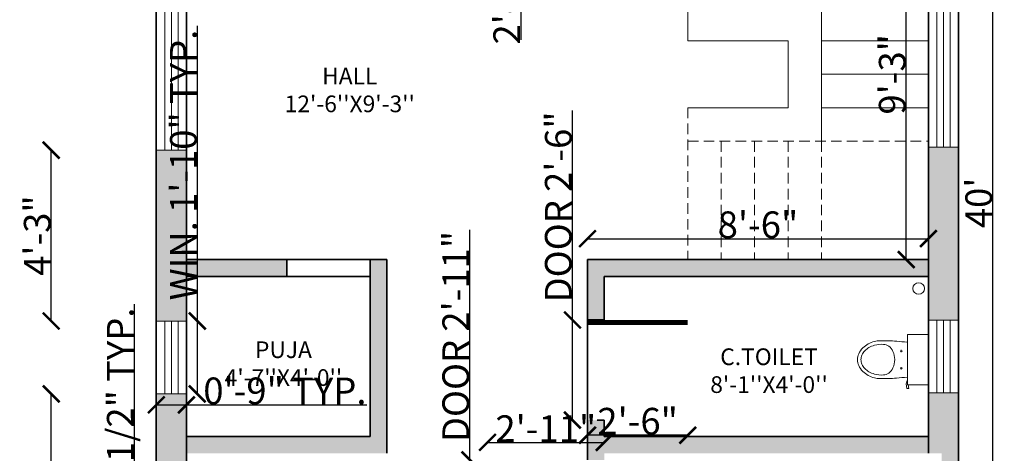
# Model space of a CAD drawing. Units: inches. Extents: x 2267 to 2908, y 1531 to 2136.
# Tile 2 of 5: x 2267 to 2562, y 1752 to 1882. Entities that reach past the tile are written whole.
import ezdxf

# ---------------------------------------------------------------- set-up
doc = ezdxf.new("R2010")
doc.units = ezdxf.units.IN
doc.linetypes.add('HIDDEN', pattern=[9.525, 6.35, -3.175])
for name, color, linetype, lineweight in [('A-ANNO-DIMS', 2, 'Continuous', 18), ('A-AREA-IDEN', 7, 'Continuous', 18), ('A-FLOR-FIXT', 9, 'Continuous', 18), ('A-FLOR-STRS-HIDN', 50, 'HIDDEN', 13), ('A-WALL-PATT', 8, 'Continuous', 13), ('DOOR', 30, 'Continuous', 18), ('STEPS', 50, 'Continuous', 18), ('WALL', 7, 'Continuous', 35), ('WINDOW', 152, 'Continuous', 18)]:
    doc.layers.add(name, color=color, linetype=linetype, lineweight=lineweight)
doc.styles.get("Standard").update_dxf_attribs({"font": 'arial.ttf'})
doc.dimstyles.get("Standard").update_dxf_attribs({"dimtxt": 8, "dimasz": 5, "dimexe": 0.18, "dimexo": 0.0625, "dimgap": 0.09, "dimtad": 1, "dimdec": 1, "dimzin": 0, "dimdsep": 46, "dimlunit": 4, "dimtxsty": 'Standard', "dimblk": 'ARCHTICK', "dimcen": 0.09, "dimse1": 1, "dimse2": 1, "dimadec": 0, "dimazin": 0, "dimtfac": 1, "dimtdec": 1, "dimtofl": 0, "dimtmove": 0, "dimatfit": 3, "dimfxl": 1, "dimtolj": 1, "dimtzin": 0, "dimarcsym": 0})

# ---------------------------------------------------------------- blocks, each defined once
blk = doc.blocks.new('A$C73484D89')
at = {"layer": 'DOOR'}
blk.add_lwpolyline([(1, 0, 0, 0, 0), (1, 0, 0, 0, 0), (0.975, 0, 0.05, 0.05, 0), (0.975, -1, 0, 0, 0), (0.95, -1, 0, 0, -0.429311), (0, 0, 0, 0, 0), (0, 0, 0, 0, 0)], format="xyseb", dxfattribs=at)
blk = doc.blocks.new('toilet-1')
at = {"color": 0, "linetype": 'ByBlock'}
for p, q in [((-0.23, -0.02), (-0.23, -0.2116)), ((0.23, -0.02), (-0.23, -0.02)), ((0.23, -0.02), (0.23, -0.2116)), ((-0.23, -0.2116), (0.23, -0.2116)), ((-0.0889, -0.2683), (-0.0697, -0.2683)), ((-0.0793, -0.2587), (-0.0793, -0.2778)), ((0.0889, -0.2683), (0.0698, -0.2683)), ((0.0794, -0.2587), (0.0794, -0.2778)), ((0.1917, -0.2144), (0.2206, -0.225)), ((0.2206, -0.225), (0.266, -0.2187)), ((0.2633, -0.1997), (0.23, -0.2044)), ((0.266, -0.2187), (0.2633, -0.1997)), ((0, -0.6382), (0, -0.6382))]:
    blk.add_line(p, q, dxfattribs=at)
for centre, radius, start, end in [((3.5272, -0.6239), 3.7093, 173.69251, 175.15926), ((-3.527, -0.624), 3.7093, 4.84131, 6.31706), ((1.7368, -0.4519), 1.9109, 175.76982, 180.37578), ((-0.0312, -0.4465), 0.1114, 113.89968, 145.1485), ((0, -0.5169), 0.1884, 66.09393, 113.90607), ((0.0312, -0.4465), 0.1114, 34.8515, 66.10032), ((-1.7366, -0.4519), 1.9109, 359.62422, 4.23018), ((0.0981, -0.4497), 0.2389, 175.88621, 195.59308), ((-0.0408, -0.4398), 0.0996, 145.14967, 175.88096), ((0.0409, -0.4398), 0.0996, 4.11904, 34.85033), ((-0.098, -0.4497), 0.2389, 344.40692, 4.11379), ((0.0353, -0.463), 0.2093, 180.37466, 194.33753), ((0.055, -0.458), 0.2297, 194.33532, 209.62204), ((0.0961, -0.4503), 0.2369, 195.59686, 209.37705), ((-0.096, -0.4503), 0.2369, 330.62295, 344.40314), ((-0.0548, -0.458), 0.2297, 330.37879, 345.66551), ((-0.0351, -0.463), 0.2093, 345.6614, 359.62427), ((0.0647, -0.4524), 0.2409, 209.62726, 224.54888), ((0.0232, -0.4913), 0.1532, 209.38715, 226.54376), ((0.0178, -0.4986), 0.1751, 224.55199, 245.714), ((0.0152, -0.4997), 0.1416, 226.55015, 246.55272), ((0, -0.5347), 0.1034, 246.54933, 270.0042), ((0, -0.5347), 0.1034, 269.9958, 293.45067), ((-0.0151, -0.4997), 0.1416, 293.44728, 313.44985), ((-0.0176, -0.4986), 0.1751, 294.28649, 315.4485), ((-0.0231, -0.4913), 0.1532, 313.45624, 330.61285), ((-0.0645, -0.4524), 0.2409, 315.45042, 330.37204), ((0.0004, -0.538), 0.132, 245.58449, 269.87817), ((-0.0002, -0.538), 0.132, 270.12162, 294.4153)]:
    blk.add_arc(centre, radius, start, end, dxfattribs=at)
blk = doc.blocks.new('_ArchTick')
at = {"color": 0, "linetype": 'ByBlock', "const_width": 0.15}
blk.add_lwpolyline([(-0.5, -0.5), (0.5, 0.5)], dxfattribs=at)
blk = doc.blocks.new('*D10')
at = {"layer": 'A-ANNO-DIMS', "color": 0, "lineweight": -2, "transparency": 16777216}
blk.add_line((2558.03, 2067.14), (2558.03, 1587.14), dxfattribs=at)
at = {"layer": 'Defpoints', "color": 0, "transparency": 16777216}
for p in [(2547.81, 2067.14), (2547.81, 1587.14), (2558.03, 1587.14)]:
    blk.add_point(p, dxfattribs=at)
at = {"layer": 'A-ANNO-DIMS', "color": 0, "lineweight": -2, "transparency": 16777216, "xscale": 5, "yscale": 5, "zscale": 5}
for p, rotation in [((2558.03, 2067.14), 90), ((2558.03, 1587.14), 270)]:
    blk.add_blockref('_ArchTick', p, dxfattribs=dict(at, rotation=rotation))
at = {"layer": 'A-ANNO-DIMS', "color": 0, "transparency": 16777216, "insert": (2553.86, 1827.14), "char_height": 8, "attachment_point": 5, "rotation": 90}
blk.add_mtext("\\A1;40'", dxfattribs=at)
blk = doc.blocks.new('*D16')
at = {"layer": 'A-ANNO-DIMS', "color": 0, "lineweight": -2, "transparency": 16777216}
blk.add_line((2436.81, 1816.42), (2538.81, 1816.42), dxfattribs=at)
at = {"layer": 'Defpoints', "color": 0, "transparency": 16777216}
for p in [(2538.81, 1816.42), (2436.81, 1810.14), (2538.81, 1810.14)]:
    blk.add_point(p, dxfattribs=at)
at = {"layer": 'A-ANNO-DIMS', "color": 0, "lineweight": -2, "transparency": 16777216, "xscale": 5, "yscale": 5, "zscale": 5, "rotation": 180}
blk.add_blockref('_ArchTick', (2436.81, 1816.42), dxfattribs=at)
at = {"layer": 'A-ANNO-DIMS', "color": 0, "lineweight": -2, "transparency": 16777216, "xscale": 5, "yscale": 5, "zscale": 5}
blk.add_blockref('_ArchTick', (2538.81, 1816.42), dxfattribs=at)
at = {"layer": 'A-ANNO-DIMS', "color": 0, "transparency": 16777216, "insert": (2487.81, 1820.59), "char_height": 8, "attachment_point": 5}
blk.add_mtext('\\A1;8\'-6"', dxfattribs=at)
blk = doc.blocks.new('*D17')
at = {"layer": 'A-ANNO-DIMS', "color": 0, "lineweight": -2, "transparency": 16777216}
blk.add_line((2532.17, 1810.14), (2532.17, 1921.14), dxfattribs=at)
at = {"layer": 'Defpoints', "color": 0, "transparency": 16777216}
for p in [(2532.17, 1921.14), (2538.81, 1921.14), (2538.81, 1810.14)]:
    blk.add_point(p, dxfattribs=at)
at = {"layer": 'A-ANNO-DIMS', "color": 0, "lineweight": -2, "transparency": 16777216, "xscale": 5, "yscale": 5, "zscale": 5}
for p, rotation in [((2532.17, 1921.14), 90), ((2532.17, 1810.14), 270)]:
    blk.add_blockref('_ArchTick', p, dxfattribs=dict(at, rotation=rotation))
at = {"layer": 'A-ANNO-DIMS', "color": 0, "transparency": 16777216, "insert": (2527.99, 1865.64), "char_height": 8, "attachment_point": 5, "rotation": 90}
blk.add_mtext('\\A1;9\'-3"', dxfattribs=at)
blk = doc.blocks.new('WIN-43_65IN')
for p, q in [((2.5, 0), (2.5, 43.65)), ((4.5, 0), (4.5, 43.65)), ((6.5, 0), (6.5, 43.65))]:
    blk.add_line(p, q)
blk.add_lwpolyline([(0, 0), (0, 43.65), (9, 43.65), (9, 0)], close=True)
blk = doc.blocks.new('WIN-21_82IN')
for p, q in [((2.5, 0), (2.5, 21.82)), ((4.5, 0), (4.5, 21.82)), ((6.5, 0), (6.5, 21.82))]:
    blk.add_line(p, q)
blk.add_lwpolyline([(0, 0), (0, 21.82), (9, 21.82), (9, 0)], close=True)
blk = doc.blocks.new('*D23')
at = {"layer": 'A-ANNO-DIMS', "color": 0, "lineweight": -2, "transparency": 16777216}
for p, q in [((2432.31, 1792.08), (2432.31, 1854.76)), ((2432.31, 1762.08), (2432.31, 1792.08))]:
    blk.add_line(p, q, dxfattribs=at)
at = {"layer": 'Defpoints', "color": 0, "transparency": 16777216}
for p in [(2432.31, 1792.08), (2436.81, 1792.08), (2436.81, 1762.08)]:
    blk.add_point(p, dxfattribs=at)
at = {"layer": 'A-ANNO-DIMS', "color": 0, "lineweight": -2, "transparency": 16777216, "xscale": 5, "yscale": 5, "zscale": 5}
for p, rotation in [((2432.31, 1792.08), 90), ((2432.31, 1762.08), 270)]:
    blk.add_blockref('_ArchTick', p, dxfattribs=dict(at, rotation=rotation))
at = {"layer": 'A-ANNO-DIMS', "color": 0, "transparency": 16777216, "insert": (2428.08, 1825.92), "char_height": 8, "attachment_point": 5, "rotation": 90}
blk.add_mtext('\\A1;DOOR 2\'-6"', dxfattribs=at)
blk = doc.blocks.new('*D24')
at = {"layer": 'A-ANNO-DIMS', "color": 0, "lineweight": -2, "transparency": 16777216}
blk.add_line((2466.81, 1757.57), (2436.81, 1757.57), dxfattribs=at)
at = {"layer": 'Defpoints', "color": 0, "transparency": 16777216}
for p in [(2436.81, 1762.08), (2466.81, 1762.08), (2436.81, 1757.57)]:
    blk.add_point(p, dxfattribs=at)
at = {"layer": 'A-ANNO-DIMS', "color": 0, "lineweight": -2, "transparency": 16777216, "xscale": 5, "yscale": 5, "zscale": 5, "rotation": 180}
blk.add_blockref('_ArchTick', (2436.81, 1757.57), dxfattribs=at)
at = {"layer": 'A-ANNO-DIMS', "color": 0, "lineweight": -2, "transparency": 16777216, "xscale": 5, "yscale": 5, "zscale": 5}
blk.add_blockref('_ArchTick', (2466.81, 1757.57), dxfattribs=at)
at = {"layer": 'A-ANNO-DIMS', "color": 0, "transparency": 16777216, "insert": (2451.81, 1761.75), "char_height": 8, "attachment_point": 5}
blk.add_mtext('\\A1;2\'-6"', dxfattribs=at)
blk = doc.blocks.new('*D25')
at = {"layer": 'A-ANNO-DIMS', "color": 0, "lineweight": -2, "transparency": 16777216}
for p, q in [((2401.63, 1750.17), (2401.63, 1819.07)), ((2401.63, 1715.22), (2401.63, 1750.17))]:
    blk.add_line(p, q, dxfattribs=at)
at = {"layer": 'Defpoints', "color": 0, "transparency": 16777216}
for p in [(2401.63, 1750.17), (2406.87, 1750.17), (2406.87, 1715.22)]:
    blk.add_point(p, dxfattribs=at)
at = {"layer": 'A-ANNO-DIMS', "color": 0, "lineweight": -2, "transparency": 16777216, "xscale": 5, "yscale": 5, "zscale": 5}
for p, rotation in [((2401.63, 1750.17), 90), ((2401.63, 1715.22), 270)]:
    blk.add_blockref('_ArchTick', p, dxfattribs=dict(at, rotation=rotation))
at = {"layer": 'A-ANNO-DIMS', "color": 0, "transparency": 16777216, "insert": (2397.4, 1787.12), "char_height": 8, "attachment_point": 5, "rotation": 90}
blk.add_mtext('\\A1;DOOR 2\'-11"', dxfattribs=at)
blk = doc.blocks.new('*D26')
at = {"layer": 'A-ANNO-DIMS', "color": 0, "lineweight": -2, "transparency": 16777216}
blk.add_line((2406.87, 1755.42), (2441.81, 1755.42), dxfattribs=at)
at = {"layer": 'Defpoints', "color": 0, "transparency": 16777216}
for p in [(2441.81, 1755.42), (2406.87, 1750.17), (2441.81, 1750.17)]:
    blk.add_point(p, dxfattribs=at)
at = {"layer": 'A-ANNO-DIMS', "color": 0, "lineweight": -2, "transparency": 16777216, "xscale": 5, "yscale": 5, "zscale": 5, "rotation": 180}
blk.add_blockref('_ArchTick', (2406.87, 1755.42), dxfattribs=at)
at = {"layer": 'A-ANNO-DIMS', "color": 0, "lineweight": -2, "transparency": 16777216, "xscale": 5, "yscale": 5, "zscale": 5}
blk.add_blockref('_ArchTick', (2441.81, 1755.42), dxfattribs=at)
at = {"layer": 'A-ANNO-DIMS', "color": 0, "transparency": 16777216, "insert": (2424.34, 1759.52), "char_height": 8, "attachment_point": 5}
blk.add_mtext('\\A1;2\'-11"', dxfattribs=at)
blk = doc.blocks.new('*D32')
at = {"layer": 'A-ANNO-DIMS', "color": 0, "lineweight": -2, "transparency": 16777216}
for p, q in [((2416.88, 1954.84), (2416.88, 1921.14)), ((2416.88, 1921.14), (2416.88, 1875.92))]:
    blk.add_line(p, q, dxfattribs=at)
at = {"layer": 'Defpoints', "color": 0, "transparency": 16777216}
for p in [(2421.94, 1954.84), (2416.88, 1921.14), (2421.94, 1921.14)]:
    blk.add_point(p, dxfattribs=at)
at = {"layer": 'A-ANNO-DIMS', "color": 0, "lineweight": -2, "transparency": 16777216, "xscale": 5, "yscale": 5, "zscale": 5}
for p, rotation in [((2416.88, 1954.84), 90), ((2416.88, 1921.14), 270)]:
    blk.add_blockref('_ArchTick', p, dxfattribs=dict(at, rotation=rotation))
at = {"layer": 'A-ANNO-DIMS', "color": 0, "transparency": 16777216, "insert": (2412.66, 1896.03), "char_height": 8, "attachment_point": 5, "rotation": 90}
blk.add_mtext('\\A1;2\'-9 1/2"', dxfattribs=at)
blk = doc.blocks.new('*D43')
at = {"layer": 'A-ANNO-DIMS', "color": 0, "lineweight": -2, "transparency": 16777216}
for p, q in [((2301.26, 1695.97), (2301.26, 1796.81)), ((2301.26, 1652.32), (2301.26, 1695.97))]:
    blk.add_line(p, q, dxfattribs=at)
at = {"layer": 'Defpoints', "color": 0, "transparency": 16777216}
for p in [(2301.26, 1695.97), (2307.81, 1695.97), (2307.81, 1652.32)]:
    blk.add_point(p, dxfattribs=at)
at = {"layer": 'A-ANNO-DIMS', "color": 0, "lineweight": -2, "transparency": 16777216, "xscale": 5, "yscale": 5, "zscale": 5}
for p, rotation in [((2301.26, 1695.97), 90), ((2301.26, 1652.32), 270)]:
    blk.add_blockref('_ArchTick', p, dxfattribs=dict(at, rotation=rotation))
at = {"layer": 'A-ANNO-DIMS', "color": 0, "transparency": 16777216, "insert": (2297.03, 1748.89), "char_height": 8, "attachment_point": 5, "rotation": 90}
blk.add_mtext('\\A1;WIN. 3\'-7 1/2" TYP.', dxfattribs=at)
blk = doc.blocks.new('*D45')
at = {"layer": 'A-ANNO-DIMS', "color": 0, "lineweight": -2, "transparency": 16777216}
for p, q in [((2320.08, 1791.76), (2320.08, 1880.18)), ((2320.08, 1769.93), (2320.08, 1791.76))]:
    blk.add_line(p, q, dxfattribs=at)
at = {"layer": 'Defpoints', "color": 0, "transparency": 16777216}
for p in [(2316.81, 1791.76), (2320.08, 1791.76), (2316.81, 1769.93)]:
    blk.add_point(p, dxfattribs=at)
at = {"layer": 'A-ANNO-DIMS', "color": 0, "lineweight": -2, "transparency": 16777216, "xscale": 5, "yscale": 5, "zscale": 5}
for p, rotation in [((2320.08, 1791.76), 90), ((2320.08, 1769.93), 270)]:
    blk.add_blockref('_ArchTick', p, dxfattribs=dict(at, rotation=rotation))
at = {"layer": 'A-ANNO-DIMS', "color": 0, "transparency": 16777216, "insert": (2315.91, 1838.47), "char_height": 8, "attachment_point": 5, "rotation": 90}
blk.add_mtext('\\A1;WIN. 1\'-10" TYP.', dxfattribs=at)
blk = doc.blocks.new('*D46')
at = {"layer": 'A-ANNO-DIMS', "color": 0, "lineweight": -2, "transparency": 16777216}
for p, q in [((2307.81, 1766.66), (2316.81, 1766.66)), ((2316.81, 1766.66), (2370.75, 1766.66))]:
    blk.add_line(p, q, dxfattribs=at)
at = {"layer": 'Defpoints', "color": 0, "transparency": 16777216}
for p in [(2307.81, 1769.93), (2316.81, 1769.93), (2316.81, 1766.66)]:
    blk.add_point(p, dxfattribs=at)
at = {"layer": 'A-ANNO-DIMS', "color": 0, "lineweight": -2, "transparency": 16777216, "xscale": 5, "yscale": 5, "zscale": 5, "rotation": 180}
blk.add_blockref('_ArchTick', (2307.81, 1766.66), dxfattribs=at)
at = {"layer": 'A-ANNO-DIMS', "color": 0, "lineweight": -2, "transparency": 16777216, "xscale": 5, "yscale": 5, "zscale": 5}
blk.add_blockref('_ArchTick', (2316.81, 1766.66), dxfattribs=at)
at = {"layer": 'A-ANNO-DIMS', "color": 0, "transparency": 16777216, "insert": (2346.28, 1770.84), "char_height": 8, "attachment_point": 5}
blk.add_mtext('\\A1;0\'-9" TYP.', dxfattribs=at)
blk = doc.blocks.new('*D55')
at = {"layer": 'A-ANNO-DIMS', "color": 0, "lineweight": -2, "transparency": 16777216}
blk.add_line((2276.36, 1695.97), (2276.36, 1769.93), dxfattribs=at)
at = {"layer": 'Defpoints', "color": 0, "transparency": 16777216}
for p in [(2276.36, 1769.93), (2307.81, 1769.93), (2307.81, 1695.97)]:
    blk.add_point(p, dxfattribs=at)
at = {"layer": 'A-ANNO-DIMS', "color": 0, "lineweight": -2, "transparency": 16777216, "xscale": 5, "yscale": 5, "zscale": 5}
for p, rotation in [((2276.36, 1769.93), 90), ((2276.36, 1695.97), 270)]:
    blk.add_blockref('_ArchTick', p, dxfattribs=dict(at, rotation=rotation))
at = {"layer": 'A-ANNO-DIMS', "color": 0, "transparency": 16777216, "insert": (2272.18, 1732.95), "char_height": 8, "attachment_point": 5, "rotation": 90}
blk.add_mtext('\\A1;6\'-2"', dxfattribs=at)
blk = doc.blocks.new('*D56')
at = {"layer": 'A-ANNO-DIMS', "color": 0, "lineweight": -2, "transparency": 16777216}
blk.add_line((2276.36, 1791.76), (2276.36, 1842.93), dxfattribs=at)
at = {"layer": 'Defpoints', "color": 0, "transparency": 16777216}
for p in [(2276.36, 1842.93), (2307.81, 1842.93), (2307.81, 1791.76)]:
    blk.add_point(p, dxfattribs=at)
at = {"layer": 'A-ANNO-DIMS', "color": 0, "lineweight": -2, "transparency": 16777216, "xscale": 5, "yscale": 5, "zscale": 5}
for p, rotation in [((2276.36, 1842.93), 90), ((2276.36, 1791.76), 270)]:
    blk.add_blockref('_ArchTick', p, dxfattribs=dict(at, rotation=rotation))
at = {"layer": 'A-ANNO-DIMS', "color": 0, "transparency": 16777216, "insert": (2272.18, 1817.34), "char_height": 8, "attachment_point": 5, "rotation": 90}
blk.add_mtext('\\A1;4\'-3"', dxfattribs=at)
blk = doc.blocks.new('*D66')
at = {"layer": 'A-ANNO-DIMS', "color": 0, "lineweight": -2, "transparency": 16777216}
blk.add_line((2900.678151, 1792.054206), (2900.678151, 1843.818992), dxfattribs=at)
at = {"layer": 'Defpoints', "color": 0, "transparency": 16777216}
for p in [(2547.807772, 1843.818992), (2900.678151, 1843.818992), (2547.807772, 1792.054206)]:
    blk.add_point(p, dxfattribs=at)
at = {"layer": 'A-ANNO-DIMS', "color": 0, "lineweight": -2, "transparency": 16777216, "xscale": 5, "yscale": 5, "zscale": 5}
for p, rotation in [((2900.678151, 1843.818992), 90), ((2900.678151, 1792.054206), 270)]:
    blk.add_blockref('_ArchTick', p, dxfattribs=dict(at, rotation=rotation))
at = {"layer": 'A-ANNO-DIMS', "color": 0, "transparency": 16777216, "insert": (2896.588151, 1817.936599), "char_height": 8, "attachment_point": 5, "rotation": 90}
blk.add_mtext('\\A1;4\'-4"', dxfattribs=at)

msp = doc.modelspace()

# ---------------------------------------------------------------- hatches: boundary and pattern name
at = {"layer": 'A-WALL-PATT', "transparency": 33554585}
h = msp.add_hatch(color=256, dxfattribs=at)
h.dxf.hatch_style = 1
h.paths.add_polyline_path([(2547.81, 2067.14), (2395.31, 2067.14), (2395.31, 2058.14), (2413.81, 2058.14), (2538.81, 2058.14), (2538.81, 2022.14), (2547.81, 2022.14)])
h.paths.add_polyline_path([(2335.31, 2067.14), (2307.81, 2067.14), (2307.81, 1992.99), (2316.81, 1992.99), (2316.81, 2058.14), (2335.31, 2058.14)])
h.paths.add_polyline_path([(2316.81, 1949.34), (2307.81, 1949.34), (2307.81, 1886.58), (2316.81, 1886.58)])
h.paths.add_polyline_path([(2316.81, 1842.93), (2307.81, 1842.93), (2307.81, 1791.76), (2316.81, 1791.76)])
h.paths.add_polyline_path([(2316.81, 1769.93), (2307.81, 1769.93), (2307.81, 1695.97), (2316.81, 1695.97)])
h.paths.add_polyline_path([(2316.81, 1652.32), (2307.81, 1652.32), (2307.81, 1587.14), (2344.81, 1587.14), (2344.81, 1596.14), (2316.81, 1596.14)])
h.paths.add_polyline_path([(2441.81, 1715.23, -0.025641), (2438.4, 1715.23), (2436.81, 1715.23), (2436.81, 1596.14), (2404.81, 1596.14), (2404.81, 1587.14), (2441.81, 1587.14)])
h.paths.add_polyline_path([(2547.81, 1770.23), (2538.81, 1770.23), (2538.81, 1752.14), (2542.81, 1752.14), (2542.81, 1587.14), (2547.81, 1587.14)])
h.paths.add_polyline_path([(2547.81, 1843.82), (2538.81, 1843.82), (2538.81, 1792.05), (2547.81, 1792.05)])
h.paths.add_polyline_path([(2547.81, 1962.14), (2538.81, 1962.14), (2538.81, 1887.47), (2547.81, 1887.47)])
h.paths.add_polyline_path([(2638.23, 1962.08), (2629.23, 1962.08), (2629.23, 1885.88), (2638.23, 1885.88)])
h.paths.add_polyline_path([(2638.23, 2056.17), (2860.23, 2056.17), (2860.23, 2020.17), (2869.23, 2020.17), (2869.23, 2065.17), (2629.23, 2065.17), (2629.23, 2022.08), (2638.23, 2022.08)])
h.paths.add_polyline_path([(2869.23, 1960.17), (2860.23, 1960.17), (2860.23, 1885.5), (2869.23, 1885.5)])
h.paths.add_polyline_path([(2869.23, 1841.85), (2860.23, 1841.85), (2860.23, 1790.08), (2869.23, 1790.08)])
h.paths.add_polyline_path([(2869.23, 1768.26), (2860.23, 1768.26), (2860.23, 1768.05), (2860.23, 1720.44), (2869.23, 1720.44)])
h.paths.add_polyline_path([(2869.23, 1660.44), (2860.23, 1660.44), (2860.23, 1585.17), (2869.23, 1585.17)])
h.paths.add_polyline_path([(2763.23, 1594.17), (2726.23, 1594.17), (2726.23, 1585.17), (2763.23, 1585.17)])
h.paths.add_polyline_path([(2666.23, 1594.17), (2638.23, 1594.17), (2638.23, 1768.3), (2629.23, 1768.3), (2629.23, 1585.17), (2666.23, 1585.17)])
h.paths.add_polyline_path([(2638.23, 1842.24), (2629.23, 1842.24), (2629.23, 1790.12), (2638.23, 1790.12)])
h = msp.add_hatch(color=256, dxfattribs=at)
h.dxf.hatch_style = 1
h.paths.add_polyline_path([(2763.23, 1755.17), (2758.23, 1755.17), (2758.23, 1625.17), (2760.21, 1625.17, -0.025641), (2763.23, 1625.17)])
h.paths.add_polyline_path([(2638.23, 1750.17), (2679.86, 1750.17, -0.025641), (2679.86, 1752.99), (2679.86, 1755.17), (2638.23, 1755.17)])
h.paths.add_polyline_path([(2860.23, 1625.17), (2860.23, 1630.17), (2796.25, 1630.17), (2796.25, 1628.39, -0.025641), (2796.25, 1625.17)])
h.paths.add_polyline_path([(2730.26, 1919.17), (2745.45, 1919.17), (2745.45, 1924.17), (2740.23, 1924.17), (2740.23, 2056.17), (2735.23, 2056.17), (2735.23, 1924.17), (2730.26, 1924.17)])
h.paths.add_polyline_path([(2860.23, 1919.17), (2860.23, 1924.17), (2774.38, 1924.17), (2774.38, 1921.99, -0.025641), (2774.38, 1919.17)])
h.paths.add_polyline_path([(2638.23, 1919.17), (2701.33, 1919.17, -0.025641), (2701.33, 1921.99), (2701.33, 1924.17), (2638.23, 1924.17)])
h.paths.add_polyline_path([(2538.81, 1752.14), (2538.81, 1757.14), (2441.81, 1757.14), (2441.81, 1762.09), (2439.73, 1762.09, -0.025641), (2436.81, 1762.09), (2436.81, 1750.17), (2441.81, 1750.17), (2441.81, 1752.14)])
h.paths.add_polyline_path([(2436.81, 1810.14), (2436.81, 1792.08), (2441.81, 1792.08), (2441.81, 1805.14), (2538.81, 1805.14), (2538.81, 1810.14)])
h.paths.add_polyline_path([(2346.81, 1805.14), (2346.81, 1810.14), (2316.81, 1810.14), (2316.81, 1805.14)], flags=0)
h.paths.add_polyline_path([(2376.81, 1810.14), (2371.81, 1810.14), (2371.81, 1757.14), (2316.81, 1757.14), (2316.81, 1752.14), (2376.81, 1752.14)])
h.paths.add_polyline_path([(2374.47, 1921.14), (2374.47, 1926.14), (2316.81, 1926.14), (2316.81, 1921.14)])
h.paths.add_polyline_path([(2413.81, 1921.14), (2421.94, 1921.14), (2421.94, 1926.14), (2418.81, 1926.14), (2418.81, 2058.14), (2413.81, 2058.14)])
h.paths.add_polyline_path([(2316.81, 2022.14), (2316.81, 2017.14), (2381.27, 2017.14), (2381.27, 2022.14)])
h.paths.add_polyline_path([(2455.63, 1926.14), (2455.63, 1924.43, -0.025641), (2455.63, 1921.14), (2538.81, 1921.14), (2538.81, 1926.14)])
h = msp.add_hatch(color=256, dxfattribs=at)
h.dxf.hatch_style = 1
h.paths.add_polyline_path([(2346.81, 1810.14), (2316.81, 1810.14), (2316.81, 1805.14), (2346.81, 1805.14)])

# ---------------------------------------------------------------- linework, layer by layer
at = {"layer": 'A-FLOR-FIXT'}
msp.add_circle((2535.9, 1801.5), 1.74, dxfattribs=at)
at = {"layer": 'A-FLOR-STRS-HIDN', "ltscale": 0.5}
for p, q in [((2466.81, 1855.64), (2466.81, 1810.14)), ((2466.81, 1845.64), (2538.81, 1845.64)), ((2476.81, 1845.64), (2476.81, 1810.14)), ((2486.81, 1845.64), (2486.81, 1810.14)), ((2496.81, 1845.64), (2496.81, 1810.14)), ((2506.81, 1845.64), (2506.81, 1810.14))]:
    msp.add_line(p, q, dxfattribs=at)
at = {"layer": 'STEPS'}
for p, q in [((2466.81, 1921.14), (2466.81, 1875.64)), ((2506.81, 1921.14), (2506.81, 1845.64)), ((2466.81, 1875.64), (2496.81, 1875.64)), ((2496.81, 1875.64), (2496.81, 1855.64)), ((2506.81, 1875.64), (2538.81, 1875.64)), ((2506.81, 1865.64), (2538.81, 1865.64)), ((2496.81, 1855.64), (2466.81, 1855.64)), ((2506.81, 1855.64), (2538.81, 1855.64))]:
    msp.add_line(p, q, dxfattribs=at)
at = {"layer": 'WALL'}
for p, q in [((2307.81, 2067.14), (2307.81, 1587.14)), ((2547.81, 2067.14), (2547.81, 1587.14)), ((2316.81, 2058.14), (2316.81, 1596.14)), ((2538.81, 2058.14), (2538.81, 1752.14)), ((2316.81, 1810.14), (2376.81, 1810.14)), ((2346.81, 1810.14), (2346.81, 1805.14)), ((2371.81, 1810.14), (2371.81, 1757.14)), ((2376.81, 1810.14), (2376.81, 1752.14)), ((2436.81, 1810.14), (2436.81, 1750.17)), ((2436.81, 1810.14), (2538.81, 1810.14)), ((2316.81, 1805.14), (2371.81, 1805.14)), ((2441.81, 1805.14), (2538.81, 1805.14)), ((2441.81, 1805.14), (2441.81, 1792.08)), ((2436.81, 1792.08), (2441.81, 1792.08)), ((2439.73, 1762.09), (2441.81, 1762.09)), ((2441.81, 1762.09), (2441.81, 1757.14)), ((2316.81, 1757.14), (2371.81, 1757.14)), ((2441.81, 1757.14), (2538.81, 1757.14))]:
    msp.add_line(p, q, dxfattribs=at)

# ---------------------------------------------------------------- block references
at = {"layer": 'A-FLOR-FIXT', "xscale": 32.64243157977233, "yscale": 32.64243157977233, "zscale": 32.64243157977233, "rotation": 270}
msp.add_blockref('toilet-1', (2539.46, 1780.19), dxfattribs=at)
at = {"layer": 'DOOR', "xscale": 29.99846110673786, "yscale": 29.99846110673786, "zscale": 29.99846110673786, "rotation": 90}
msp.add_blockref('A$C73484D89', (2436.81, 1762.09), dxfattribs=at)
at = {"layer": 'WINDOW'}
for name, p in [('WIN-43_65IN', (2307.81, 1842.93)), ('WIN-43_65IN', (2538.81, 1843.82)), ('WIN-21_82IN', (2307.81, 1769.93)), ('WIN-21_82IN', (2538.81, 1770.23))]:
    msp.add_blockref(name, p, dxfattribs=at)

# ---------------------------------------------------------------- texts
at = {"layer": 'A-AREA-IDEN', "char_height": 5, "attachment_point": 1}
for s, insert in [("\\pxqc;HALL\\P12'-6''X9'-3''", (2344.98, 1867.62)), ("\\pxqc;PUJA\\P4'-7''X4'-0''", (2325.14, 1785.67)), ("\\pxqc;C.TOILET\\P8'-1''X4'-0''", (2470.42, 1783.56))]:
    msp.add_mtext_dynamic_manual_height_columns(s, width=41.4104, gutter_width=12.5, heights=[0], dxfattribs=dict(at, insert=insert))

# ---------------------------------------------------------------- dimensions: what is measured, and where the dimension line sits
at = {"layer": 'A-ANNO-DIMS'}
for base, p1, p2, angle, override, picture, middle in [((2558.03, 1587.14), (2547.81, 2067.14), (2547.81, 1587.14), 90, {"dimclrd": 0, "dimclre": 0, "dimclrt": 0}, '*D10', (2553.86, 1827.14)), ((2416.88, 1921.14), (2421.94, 1954.84), (2421.94, 1921.14), 270, {"dimdec": 1, "dimlfac": 1, "dimrnd": 0, "dimzin": 1, "dimdsep": 46, "dimlunit": 4, "dimfrac": 2}, '*D32', (2412.66, 1896.03)), ((2532.17, 1921.14), (2538.81, 1810.14), (2538.81, 1921.14), 90, {"dimclrd": 0, "dimclre": 0, "dimclrt": 0}, '*D17', (2527.99, 1865.64)), ((2276.36, 1842.93), (2307.81, 1791.76), (2307.81, 1842.93), 90, {"dimdec": 1, "dimlfac": 1, "dimrnd": 0, "dimzin": 1, "dimdsep": 46, "dimlunit": 4, "dimfrac": 2}, '*D56', (2272.18, 1817.34)), ((2900.68, 1843.82), (2547.81, 1792.05), (2547.81, 1843.82), 90, {"dimdec": 1, "dimlfac": 1, "dimrnd": 0, "dimzin": 1, "dimdsep": 46, "dimlunit": 4, "dimfrac": 2}, '*D66', (2896.59, 1817.94)), ((2276.36, 1769.93), (2307.81, 1695.97), (2307.81, 1769.93), 90, {"dimdec": 1, "dimlfac": 1, "dimrnd": 0, "dimzin": 1, "dimdsep": 46, "dimlunit": 4, "dimfrac": 2}, '*D55', (2272.18, 1732.95)), ((2436.81, 1757.57), (2466.81, 1762.08), (2436.81, 1762.08), 180, {"dimdec": 1, "dimlfac": 1, "dimrnd": 0, "dimzin": 1, "dimdsep": 46, "dimlunit": 4, "dimfrac": 2}, '*D24', (2451.81, 1761.75))]:
    dim = msp.add_linear_dim(base=base, p1=p1, p2=p2, angle=angle, dimstyle='Standard', override=override, dxfattribs=at)
    dim.commit()
    dim.dimension.update_dxf_attribs({"geometry": picture, "text_midpoint": middle})
for base, p1, p2, text, picture, middle in [((2320.08, 1791.76), (2316.81, 1769.93), (2316.81, 1791.76), 'WIN. <> TYP.', '*D45', (2315.91, 1838.47)), ((2432.31, 1792.08), (2436.81, 1762.08), (2436.81, 1792.08), 'DOOR <>', '*D23', (2428.08, 1825.92)), ((2401.6262, 1750.1728), (2406.8687, 1715.2225), (2406.8687, 1750.1728), 'DOOR <>', '*D25', (2397.397, 1787.1209)), ((2301.2607, 1695.9659), (2307.8078, 1652.319), (2307.8078, 1695.9659), 'WIN. <> TYP.', '*D43', (2297.0316, 1748.8895))]:
    dim = msp.add_linear_dim(base=base, p1=p1, p2=p2, angle=90, text=text, dimstyle='Standard', override={"dimdec": 1, "dimlfac": 1, "dimrnd": 0, "dimzin": 1, "dimdsep": 46, "dimlunit": 4, "dimfrac": 2}, dxfattribs=at)
    dim.commit()
    dim.dimension.update_dxf_attribs({"geometry": picture, "text_midpoint": middle})
for base, p1, p2, override, picture, middle in [((2538.81, 1816.42), (2436.81, 1810.14), (2538.81, 1810.14), {"dimclrd": 0, "dimclre": 0, "dimclrt": 0}, '*D16', (2487.81, 1820.59)), ((2441.81, 1755.42), (2406.87, 1750.17), (2441.81, 1750.17), {"dimdec": 1, "dimlfac": 1, "dimrnd": 0, "dimzin": 1, "dimdsep": 46, "dimlunit": 4, "dimfrac": 2}, '*D26', (2424.34, 1759.52))]:
    dim = msp.add_linear_dim(base=base, p1=p1, p2=p2, dimstyle='Standard', override=override, dxfattribs=at)
    dim.commit()
    dim.dimension.update_dxf_attribs({"geometry": picture, "text_midpoint": middle})
dim = msp.add_linear_dim(base=(2316.81, 1766.66), p1=(2307.81, 1769.93), p2=(2316.81, 1769.93), text='<> TYP.', dimstyle='Standard', override={"dimdec": 1, "dimlfac": 1, "dimrnd": 0, "dimzin": 1, "dimdsep": 46, "dimlunit": 4, "dimfrac": 2}, dxfattribs=at)
dim.commit()
dim.dimension.update_dxf_attribs({"geometry": '*D46', "text_midpoint": (2346.28, 1770.84)})

doc.saveas('drawing.dxf')
